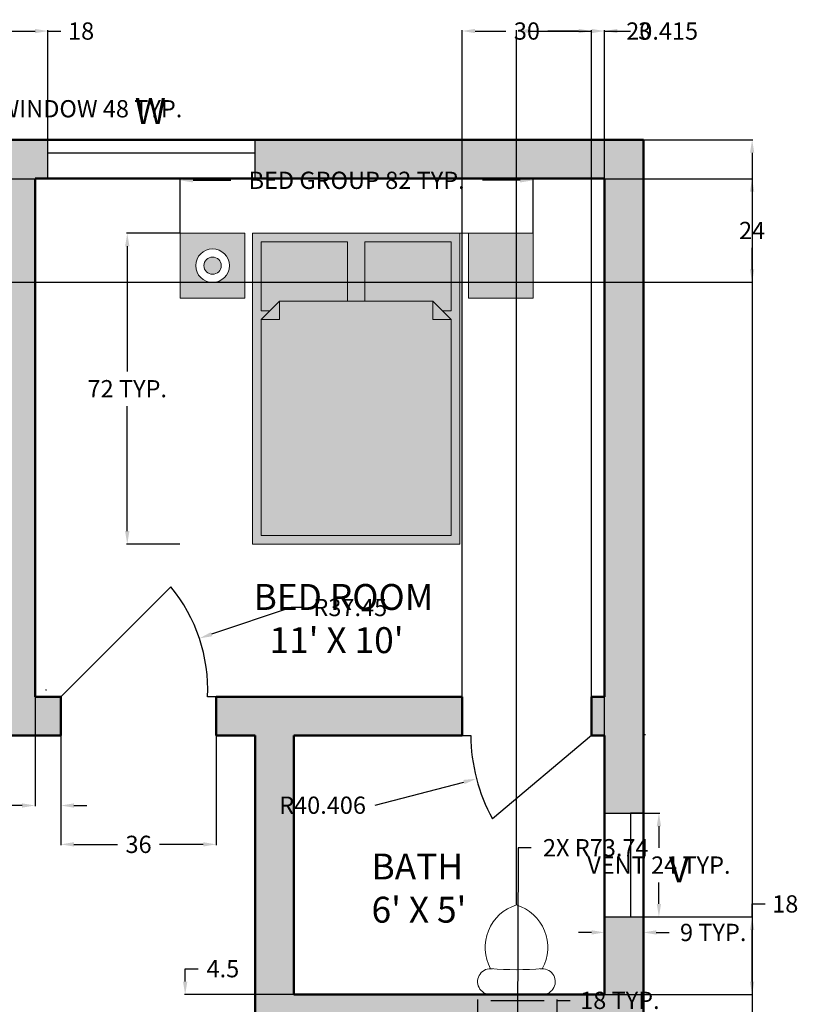
# Model space of a CAD drawing. Units: inches. Extents: x 30 to 385, y 81 to 626.
# Tile 4 of 4: x 204 to 385, y 398 to 626. Entities that reach past the tile are written whole.
import ezdxf

# ---------------------------------------------------------------- set-up
doc = ezdxf.new("R2010")
doc.units = ezdxf.units.IN
doc.header["$MEASUREMENT"] = 0
for name, color, linetype, lineweight in [('A-ANNO-DIMS', 2, 'Continuous', 18), ('A-ANNO-TEXT', 7, 'Continuous', 18), ('A-AREA-IDEN', 7, 'Continuous', 25), ('A-DOOR', 3, 'Continuous', 25), ('A-FLOR-FIXT', 8, 'Continuous', 18), ('A-FURN', 8, 'Continuous', 18), ('A-GLAZ', 4, 'Continuous', 25), ('A-WALL', 7, 'Continuous', 50), ('A-WALL-PATT', 32, 'Continuous', 13)]:
    doc.layers.add(name, color=color, linetype=linetype, lineweight=lineweight)
doc.layers.add('A-FURN-PATT', color=254, linetype='Continuous', lineweight=13, true_color=0xfeeab9)
doc.styles.get("Standard").update_dxf_attribs({"font": 'arial.ttf'})
doc.dimstyles.get("Standard").update_dxf_attribs({"dimtxt": 4, "dimasz": 3, "dimexe": 0.18, "dimexo": 0.0625, "dimgap": 2, "dimtad": 0, "dimtih": 1, "dimtoh": 1, "dimdec": 0, "dimzin": 0, "dimdsep": 46, "dimlunit": 3, "dimtxsty": 'Standard', "dimcen": 0.09, "dimadec": 0, "dimazin": 0, "dimtfac": 1, "dimtdec": 0, "dimtofl": 0, "dimtmove": 0, "dimatfit": 3, "dimfxl": 1, "dimtolj": 1, "dimtzin": 0, "dimarcsym": 0})

# ---------------------------------------------------------------- blocks, each defined once
blk = doc.blocks.new('WIN-48')
for p, q in [((0, 0), (0, 9)), ((48, 0), (48, 9)), ((0, 6), (48, 6))]:
    blk.add_line(p, q)
blk = doc.blocks.new('VENT-24')
for p, q in [((0, 0), (9, 0)), ((6, 0), (6, -24)), ((0, -24), (9, -24))]:
    blk.add_line(p, q)
blk = doc.blocks.new('WC-TANK')
blk.add_line((0, 0), (-12, 0.05))
for centre, radius, start, end in [((-12.01, -2.95), 3, 89.7749, 278.744), ((-0.01, -3), 3, 260.8057, 89.7749), ((-3.03, -10.92), 10.27, 151.067, 252.7388), ((-6.31, -79.48), 73.74, 85.108, 94.4417), ((-9.05, -10.9), 10.27, 286.8109, 28.4828)]:
    blk.add_arc(centre, radius, start, end)
blk = doc.blocks.new('BED-48X72-WITH-NIGHTSTANDS')
for p, q in [((48, 0), (50, 0)), ((2, -2), (22, -2)), ((2, -18), (2, -2)), ((22, -2), (22, -15.76)), ((26, -2), (46, -2)), ((26, -2), (26, -15.76)), ((46, -2), (46, -18)), ((2, -20), (6.24, -15.76)), ((41.76, -15.76), (6.24, -15.76)), ((6.24, -15.76), (6.24, -20)), ((46, -20), (41.76, -15.76)), ((41.76, -15.76), (41.76, -20)), ((2, -18), (4, -18)), ((44, -18), (46, -18)), ((2, -20), (6.24, -20)), ((2, -70), (2, -20)), ((41.76, -20), (46, -20)), ((46, -20), (46, -70)), ((46, -70), (2, -70))]:
    blk.add_line(p, q)
for points in [[(-16.78, 0), (-1.78, 0), (-1.78, -15), (-16.78, -15)], [(0, 0), (48, 0), (48, -72), (0, -72)], [(50, 0), (65, 0), (65, -15), (50, -15)]]:
    blk.add_lwpolyline(points, close=True)
for radius in [3.89, 3.89, 3.89, 2]:
    blk.add_circle((-9.28, -7.5), radius)
blk = doc.blocks.new('*D6')
at = {"layer": 'A-ANNO-DIMS', "color": 0, "lineweight": -2, "transparency": 16777216}
for p, q in [((144.92, 598.13), (144.92, 605.44)), ((147.92, 605.26), (189.92, 605.26)), ((192.92, 598.13), (192.92, 605.44)), ((192.92, 605.26), (195.92, 605.26))]:
    blk.add_line(p, q, dxfattribs=at)
at = {"layer": 'A-ANNO-DIMS', "color": 0, "transparency": 16777216}
for points in [[(147.92, 605.76), (147.92, 604.76), (144.92, 605.26)], [(189.92, 605.76), (189.92, 604.76), (192.92, 605.26)]]:
    blk.add_solid(points, dxfattribs=at)
at = {"layer": 'Defpoints', "color": 0, "transparency": 16777216}
for p in [(192.92, 605.26), (144.92, 598.06), (192.92, 598.06)]:
    blk.add_point(p, dxfattribs=at)
at = {"layer": 'A-ANNO-DIMS', "color": 0, "transparency": 16777216, "insert": (220.77, 605.26), "char_height": 4, "attachment_point": 5}
blk.add_mtext('\\A1;WINDOW 48 TYP.', dxfattribs=at)
blk = doc.blocks.new('*D8')
at = {"layer": 'A-ANNO-DIMS', "color": 0, "lineweight": -2, "transparency": 16777216}
for p, q in [((348.98, 442.06), (352.7, 442.06)), ((352.52, 439.06), (352.52, 434.07)), ((352.52, 421.06), (352.52, 426.05)), ((348.98, 418.06), (352.7, 418.06))]:
    blk.add_line(p, q, dxfattribs=at)
at = {"layer": 'A-ANNO-DIMS', "color": 0, "transparency": 16777216}
for points in [[(352.02, 439.06), (353.02, 439.06), (352.52, 442.06)], [(352.02, 421.06), (353.02, 421.06), (352.52, 418.06)]]:
    blk.add_solid(points, dxfattribs=at)
at = {"layer": 'Defpoints', "color": 0, "transparency": 16777216}
for p in [(348.92, 442.06), (352.52, 442.06), (348.92, 418.06)]:
    blk.add_point(p, dxfattribs=at)
at = {"layer": 'A-ANNO-DIMS', "color": 0, "transparency": 16777216, "insert": (352.52, 430.06), "char_height": 4, "attachment_point": 5}
blk.add_mtext('\\A1;VENT 24 TYP.', dxfattribs=at)
blk = doc.blocks.new('*D9')
at = {"layer": 'A-ANNO-DIMS', "color": 0, "lineweight": -2, "transparency": 16777216}
for p, q in [((339.92, 418), (339.92, 414.28)), ((348.92, 418), (348.92, 414.28)), ((336.92, 414.46), (333.92, 414.46)), ((351.92, 414.46), (354.92, 414.46))]:
    blk.add_line(p, q, dxfattribs=at)
at = {"layer": 'A-ANNO-DIMS', "color": 0, "transparency": 16777216}
for points in [[(336.92, 414.96), (336.92, 413.96), (339.92, 414.46)], [(351.92, 414.96), (351.92, 413.96), (348.92, 414.46)]]:
    blk.add_solid(points, dxfattribs=at)
at = {"layer": 'Defpoints', "color": 0, "transparency": 16777216}
for p in [(339.92, 418.06), (348.92, 418.06), (348.92, 414.46)]:
    blk.add_point(p, dxfattribs=at)
at = {"layer": 'A-ANNO-DIMS', "color": 0, "transparency": 16777216, "insert": (365.1, 414.46), "char_height": 4, "attachment_point": 5}
blk.add_mtext('\\A1;9 TYP.', dxfattribs=at)
blk = doc.blocks.new('*D11')
at = {"layer": 'A-ANNO-DIMS', "color": 0, "lineweight": -2, "transparency": 16777216}
for p, q in [((310.55, 395.68), (310.55, 398.91)), ((313.55, 398.73), (325.92, 398.73)), ((328.92, 395.68), (328.92, 398.91)), ((328.92, 398.73), (331.92, 398.73))]:
    blk.add_line(p, q, dxfattribs=at)
at = {"layer": 'A-ANNO-DIMS', "color": 0, "transparency": 16777216}
for points in [[(313.55, 399.23), (313.55, 398.23), (310.55, 398.73)], [(325.92, 399.23), (325.92, 398.23), (328.92, 398.73)]]:
    blk.add_solid(points, dxfattribs=at)
at = {"layer": 'Defpoints', "color": 0, "transparency": 16777216}
for p in [(328.92, 398.73), (310.55, 395.62), (328.92, 395.62)]:
    blk.add_point(p, dxfattribs=at)
at = {"layer": 'A-ANNO-DIMS', "color": 0, "transparency": 16777216, "insert": (343.47, 398.73), "char_height": 4, "attachment_point": 5}
blk.add_mtext('\\A1;18 TYP.', dxfattribs=at)
blk = doc.blocks.new('*D12')
at = {"layer": 'A-ANNO-DIMS', "color": 0, "lineweight": -2, "transparency": 16777216}
for p, q in [((241.57, 576.47), (241.57, 588.86)), ((244.57, 588.68), (253.27, 588.68)), ((320.35, 588.68), (311.65, 588.68)), ((323.35, 576.47), (323.35, 588.86))]:
    blk.add_line(p, q, dxfattribs=at)
at = {"layer": 'A-ANNO-DIMS', "color": 0, "transparency": 16777216}
for points in [[(244.57, 589.18), (244.57, 588.18), (241.57, 588.68)], [(320.35, 589.18), (320.35, 588.18), (323.35, 588.68)]]:
    blk.add_solid(points, dxfattribs=at)
at = {"layer": 'Defpoints', "color": 0, "transparency": 16777216}
for p in [(323.35, 588.68), (241.57, 576.41), (323.35, 576.41)]:
    blk.add_point(p, dxfattribs=at)
at = {"layer": 'A-ANNO-DIMS', "color": 0, "transparency": 16777216, "insert": (282.46, 588.68), "char_height": 4, "attachment_point": 5}
blk.add_mtext('\\A1;BED GROUP 82 TYP.', dxfattribs=at)
blk = doc.blocks.new('*D13')
at = {"layer": 'A-ANNO-DIMS', "color": 0, "lineweight": -2, "transparency": 16777216}
for p, q in [((241.51, 576.41), (229.12, 576.41)), ((229.3, 573.41), (229.3, 544.42)), ((229.3, 507.41), (229.3, 536.4)), ((241.51, 504.41), (229.12, 504.41))]:
    blk.add_line(p, q, dxfattribs=at)
at = {"layer": 'A-ANNO-DIMS', "color": 0, "transparency": 16777216}
for points in [[(228.8, 573.41), (229.8, 573.41), (229.3, 576.41)], [(228.8, 507.41), (229.8, 507.41), (229.3, 504.41)]]:
    blk.add_solid(points, dxfattribs=at)
at = {"layer": 'Defpoints', "color": 0, "transparency": 16777216}
for p in [(229.3, 576.41), (241.57, 576.41), (241.57, 504.41)]:
    blk.add_point(p, dxfattribs=at)
at = {"layer": 'A-ANNO-DIMS', "color": 0, "transparency": 16777216, "insert": (229.3, 540.41), "char_height": 4, "attachment_point": 5}
blk.add_mtext('\\A1;72 TYP.', dxfattribs=at)
blk = doc.blocks.new('*D17')
at = {"layer": 'A-ANNO-DIMS', "color": 0, "lineweight": -2, "transparency": 16777216}
for p, q in [((348.98, 598.06), (374.3, 598.06)), ((374.12, 595.06), (374.12, 357.61)), ((374.12, 112.06), (374.12, 349.52)), ((348.98, 109.06), (374.3, 109.06))]:
    blk.add_line(p, q, dxfattribs=at)
at = {"layer": 'A-ANNO-DIMS', "color": 0, "transparency": 16777216}
for points in [[(373.62, 595.06), (374.62, 595.06), (374.12, 598.06)], [(373.62, 112.06), (374.62, 112.06), (374.12, 109.06)]]:
    blk.add_solid(points, dxfattribs=at)
at = {"layer": 'Defpoints', "color": 0, "transparency": 16777216}
for p in [(348.92, 598.06), (374.12, 598.06), (348.92, 109.06)]:
    blk.add_point(p, dxfattribs=at)
at = {"layer": 'A-ANNO-DIMS', "color": 0, "transparency": 16777216, "insert": (374.12, 353.56), "char_height": 4, "attachment_point": 5}
blk.add_mtext('\\A1;489', dxfattribs=at)
blk = doc.blocks.new('*D22')
at = {"layer": 'A-ANNO-DIMS', "color": 0, "lineweight": -2, "transparency": 16777216}
for p, q in [((374.12, 418.06), (374.12, 421.06)), ((374.12, 421.06), (377.12, 421.06)), ((339.98, 418.06), (374.3, 418.06)), ((374.12, 403.06), (374.12, 415.06)), ((339.98, 400.06), (374.3, 400.06))]:
    blk.add_line(p, q, dxfattribs=at)
at = {"layer": 'A-ANNO-DIMS', "color": 0, "transparency": 16777216}
for points in [[(373.62, 415.06), (374.62, 415.06), (374.12, 418.06)], [(373.62, 403.06), (374.62, 403.06), (374.12, 400.06)]]:
    blk.add_solid(points, dxfattribs=at)
at = {"layer": 'Defpoints', "color": 0, "transparency": 16777216}
for p in [(339.92, 418.06), (374.12, 418.06), (339.92, 400.06)]:
    blk.add_point(p, dxfattribs=at)
at = {"layer": 'A-ANNO-DIMS', "color": 0, "transparency": 16777216, "insert": (381.8, 421.06), "char_height": 4, "attachment_point": 5}
blk.add_mtext('\\A1;18', dxfattribs=at)
blk = doc.blocks.new('*D27')
at = {"layer": 'A-ANNO-DIMS', "color": 0, "lineweight": -2, "transparency": 16777216}
for p, q in [((192.92, 598.13), (192.92, 623.44)), ((195.92, 623.26), (207.92, 623.26)), ((210.92, 598.13), (210.92, 623.44)), ((210.92, 623.26), (213.92, 623.26))]:
    blk.add_line(p, q, dxfattribs=at)
at = {"layer": 'A-ANNO-DIMS', "color": 0, "transparency": 16777216}
for points in [[(195.92, 623.76), (195.92, 622.76), (192.92, 623.26)], [(207.92, 623.76), (207.92, 622.76), (210.92, 623.26)]]:
    blk.add_solid(points, dxfattribs=at)
at = {"layer": 'Defpoints', "color": 0, "transparency": 16777216}
for p in [(210.92, 623.26), (192.92, 598.06), (210.92, 598.06)]:
    blk.add_point(p, dxfattribs=at)
at = {"layer": 'A-ANNO-DIMS', "color": 0, "transparency": 16777216, "insert": (218.6, 623.26), "char_height": 4, "attachment_point": 5}
blk.add_mtext('\\A1;18', dxfattribs=at)
blk = doc.blocks.new('*D29')
at = {"layer": 'A-ANNO-DIMS', "color": 0, "lineweight": -2, "transparency": 16777216}
for p, q in [((198.98, 589.06), (374.3, 589.06)), ((374.12, 586.06), (374.12, 581.07)), ((374.12, 568.06), (374.12, 573.06)), ((198.98, 565.06), (374.3, 565.06))]:
    blk.add_line(p, q, dxfattribs=at)
at = {"layer": 'A-ANNO-DIMS', "color": 0, "transparency": 16777216}
for points in [[(373.62, 586.06), (374.62, 586.06), (374.12, 589.06)], [(373.62, 568.06), (374.62, 568.06), (374.12, 565.06)]]:
    blk.add_solid(points, dxfattribs=at)
at = {"layer": 'Defpoints', "color": 0, "transparency": 16777216}
for p in [(198.92, 589.06), (374.12, 589.06), (198.92, 565.06)]:
    blk.add_point(p, dxfattribs=at)
at = {"layer": 'A-ANNO-DIMS', "color": 0, "transparency": 16777216, "insert": (374.12, 577.06), "char_height": 4, "attachment_point": 5}
blk.add_mtext('\\A1;24', dxfattribs=at)
blk = doc.blocks.new('*D34')
at = {"layer": 'A-ANNO-DIMS', "color": 0, "lineweight": -2, "transparency": 16777216}
for p, q in [((213.92, 460), (213.92, 434.68)), ((249.92, 460), (249.92, 434.68)), ((216.92, 434.86), (227.06, 434.86)), ((246.92, 434.86), (236.78, 434.86))]:
    blk.add_line(p, q, dxfattribs=at)
at = {"layer": 'A-ANNO-DIMS', "color": 0, "transparency": 16777216}
for points in [[(216.92, 435.36), (216.92, 434.36), (213.92, 434.86)], [(246.92, 435.36), (246.92, 434.36), (249.92, 434.86)]]:
    blk.add_solid(points, dxfattribs=at)
at = {"layer": 'Defpoints', "color": 0, "transparency": 16777216}
for p in [(213.92, 460.06), (249.92, 460.06), (213.92, 434.86)]:
    blk.add_point(p, dxfattribs=at)
at = {"layer": 'A-ANNO-DIMS', "color": 0, "transparency": 16777216, "insert": (231.92, 434.86), "char_height": 4, "attachment_point": 5}
blk.add_mtext('\\A1;36', dxfattribs=at)
blk = doc.blocks.new('*D35')
at = {"layer": 'A-ANNO-DIMS', "color": 0, "lineweight": -2, "transparency": 16777216}
for p, q in [((207.92, 469), (207.92, 443.68)), ((213.92, 469), (213.92, 443.68)), ((204.92, 443.86), (201.92, 443.86)), ((216.92, 443.86), (219.92, 443.86))]:
    blk.add_line(p, q, dxfattribs=at)
at = {"layer": 'A-ANNO-DIMS', "color": 0, "transparency": 16777216}
for points in [[(204.92, 444.36), (204.92, 443.36), (207.92, 443.86)], [(216.92, 444.36), (216.92, 443.36), (213.92, 443.86)]]:
    blk.add_solid(points, dxfattribs=at)
at = {"layer": 'Defpoints', "color": 0, "transparency": 16777216}
for p in [(207.92, 469.06), (213.92, 469.06), (207.92, 443.86)]:
    blk.add_point(p, dxfattribs=at)
at = {"layer": 'A-ANNO-DIMS', "color": 0, "transparency": 16777216, "insert": (198.6, 443.86), "char_height": 4, "attachment_point": 5}
blk.add_mtext('\\A1;6', dxfattribs=at)
blk = doc.blocks.new('*D38')
at = {"layer": 'A-ANNO-DIMS', "color": 0, "lineweight": -2, "transparency": 16777216}
for p, q in [((306.92, 460.13), (306.92, 623.44)), ((309.92, 623.26), (317.06, 623.26)), ((333.92, 623.26), (326.78, 623.26)), ((336.92, 460.13), (336.92, 623.44))]:
    blk.add_line(p, q, dxfattribs=at)
at = {"layer": 'A-ANNO-DIMS', "color": 0, "transparency": 16777216}
for points in [[(309.92, 623.76), (309.92, 622.76), (306.92, 623.26)], [(333.92, 623.76), (333.92, 622.76), (336.92, 623.26)]]:
    blk.add_solid(points, dxfattribs=at)
at = {"layer": 'Defpoints', "color": 0, "transparency": 16777216}
for p in [(336.92, 623.26), (306.92, 460.06), (336.92, 460.06)]:
    blk.add_point(p, dxfattribs=at)
at = {"layer": 'A-ANNO-DIMS', "color": 0, "transparency": 16777216, "insert": (321.92, 623.26), "char_height": 4, "attachment_point": 5}
blk.add_mtext('\\A1;30', dxfattribs=at)
blk = doc.blocks.new('*D39')
at = {"layer": 'A-ANNO-DIMS', "color": 0, "lineweight": -2, "transparency": 16777216}
for p, q in [((333.92, 623.26), (330.92, 623.26)), ((336.92, 460.13), (336.92, 623.44)), ((339.92, 460.13), (339.92, 623.44)), ((342.92, 623.26), (345.92, 623.26))]:
    blk.add_line(p, q, dxfattribs=at)
at = {"layer": 'A-ANNO-DIMS', "color": 0, "transparency": 16777216}
for points in [[(333.92, 623.76), (333.92, 622.76), (336.92, 623.26)], [(342.92, 623.76), (342.92, 622.76), (339.92, 623.26)]]:
    blk.add_solid(points, dxfattribs=at)
at = {"layer": 'Defpoints', "color": 0, "transparency": 16777216}
for p in [(339.92, 623.26), (336.92, 460.06), (339.92, 460.06)]:
    blk.add_point(p, dxfattribs=at)
at = {"layer": 'A-ANNO-DIMS', "color": 0, "transparency": 16777216, "insert": (349.23, 623.26), "char_height": 4, "attachment_point": 5}
blk.add_mtext('\\A1;3', dxfattribs=at)
blk = doc.blocks.new('*D41')
at = {"layer": 'A-ANNO-DIMS', "color": 0, "lineweight": -2, "transparency": 16777216}
for p, q in [((242.72, 403.06), (242.72, 406.06)), ((242.72, 406.06), (245.72, 406.06)), ((267.86, 400.06), (242.54, 400.06)), ((267.86, 395.56), (242.54, 395.56)), ((242.72, 392.56), (242.72, 389.56))]:
    blk.add_line(p, q, dxfattribs=at)
at = {"layer": 'A-ANNO-DIMS', "color": 0, "transparency": 16777216}
for points in [[(242.22, 403.06), (243.22, 403.06), (242.72, 400.06)], [(242.22, 392.56), (243.22, 392.56), (242.72, 395.56)]]:
    blk.add_solid(points, dxfattribs=at)
at = {"layer": 'Defpoints', "color": 0, "transparency": 16777216}
for p in [(242.72, 400.06), (267.92, 400.06), (267.92, 395.56)]:
    blk.add_point(p, dxfattribs=at)
at = {"layer": 'A-ANNO-DIMS', "color": 0, "transparency": 16777216, "insert": (251.46, 406.06), "char_height": 4, "attachment_point": 5}
blk.add_mtext('\\A1;4.5', dxfattribs=at)
blk = doc.blocks.new('*D42')
at = {"layer": 'A-ANNO-DIMS', "color": 0, "lineweight": -2, "transparency": 16777216}
for p, q in [((319.5, 420.88), (319.5, 623.44)), ((322.5, 623.26), (336.92, 623.26)), ((339.92, 418.13), (339.92, 623.44)), ((339.92, 623.26), (342.92, 623.26))]:
    blk.add_line(p, q, dxfattribs=at)
at = {"layer": 'A-ANNO-DIMS', "color": 0, "transparency": 16777216}
for points in [[(322.5, 623.76), (322.5, 622.76), (319.5, 623.26)], [(336.92, 623.76), (336.92, 622.76), (339.92, 623.26)]]:
    blk.add_solid(points, dxfattribs=at)
at = {"layer": 'Defpoints', "color": 0, "transparency": 16777216}
for p in [(339.92, 623.26), (319.5, 420.82), (339.92, 418.06)]:
    blk.add_point(p, dxfattribs=at)
at = {"layer": 'A-ANNO-DIMS', "color": 0, "transparency": 16777216, "insert": (353.27, 623.26), "char_height": 4, "attachment_point": 5}
blk.add_mtext('\\A1;20.415', dxfattribs=at)
blk = doc.blocks.new('*D56')
at = {"layer": 'A-ANNO-DIMS', "color": 0, "lineweight": -2, "transparency": 16777216}
for p, q in [((267.31, 489.73), (248.85, 483.54)), ((270.31, 489.73), (267.31, 489.73)), ((210.41, 470.67), (210.59, 470.67)), ((210.5, 470.58), (210.5, 470.76))]:
    blk.add_line(p, q, dxfattribs=at)
at = {"layer": 'A-ANNO-DIMS', "color": 0, "transparency": 16777216}
blk.add_solid([(248.69, 484.01), (249.01, 483.06), (246.01, 482.58)], dxfattribs=at)
at = {"layer": 'Defpoints', "color": 0, "transparency": 16777216}
for p in [(246.01, 482.58), (210.5, 470.67)]:
    blk.add_point(p, dxfattribs=at)
at = {"layer": 'A-ANNO-DIMS', "color": 0, "transparency": 16777216, "insert": (280.99, 489.73), "char_height": 4, "attachment_point": 5}
blk.add_mtext('\\A1;R37.45', dxfattribs=at)
blk = doc.blocks.new('*D58')
at = {"layer": 'A-ANNO-DIMS', "color": 0, "lineweight": -2, "transparency": 16777216}
for p, q in [((349.23, 460.28), (349.41, 460.28)), ((349.32, 460.19), (349.32, 460.37)), ((286.78, 443.93), (307.33, 449.3))]:
    blk.add_line(p, q, dxfattribs=at)
at = {"layer": 'A-ANNO-DIMS', "color": 0, "transparency": 16777216}
blk.add_solid([(307.2, 449.79), (307.46, 448.82), (310.23, 450.06)], dxfattribs=at)
at = {"layer": 'Defpoints', "color": 0, "transparency": 16777216}
for p in [(349.32, 460.28), (310.23, 450.06)]:
    blk.add_point(p, dxfattribs=at)
at = {"layer": 'A-ANNO-DIMS', "color": 0, "transparency": 16777216, "insert": (274.56, 443.93), "char_height": 4, "attachment_point": 5}
blk.add_mtext('\\A1;R40.406', dxfattribs=at)
blk = doc.blocks.new('*D59')
at = {"layer": 'A-ANNO-DIMS', "color": 0, "lineweight": -2, "transparency": 16777216}
for p, q in [((319.9, 434.08), (319.73, 392.83)), ((322.9, 434.08), (319.9, 434.08)), ((319.34, 316.09), (319.52, 316.09)), ((319.43, 316), (319.43, 316.18))]:
    blk.add_line(p, q, dxfattribs=at)
at = {"layer": 'A-ANNO-DIMS', "color": 0, "transparency": 16777216}
blk.add_solid([(319.23, 392.83), (320.23, 392.83), (319.72, 389.83)], dxfattribs=at)
at = {"layer": 'Defpoints', "color": 0, "transparency": 16777216}
for p in [(319.72, 389.83), (319.43, 316.09)]:
    blk.add_point(p, dxfattribs=at)
at = {"layer": 'A-ANNO-DIMS', "color": 0, "transparency": 16777216, "insert": (337.88, 434.08), "char_height": 4, "attachment_point": 5}
blk.add_mtext('\\A1;2X R73.74', dxfattribs=at)

msp = doc.modelspace()

# ---------------------------------------------------------------- hatches: boundary and pattern name
at = {"layer": 'A-FURN-PATT'}
h = msp.add_hatch(color=256, dxfattribs=at)
h.paths.add_polyline_path([(306.3516, 576.4124), (258.3516, 576.4124), (258.3516, 504.4124), (306.3516, 504.4124)])
h.paths.add_polyline_path([(260.3516, 558.4124), (260.3516, 574.4124), (280.3516, 574.4124), (280.3516, 560.655), (284.3516, 560.655), (284.3516, 574.4124), (304.3516, 574.4124), (304.3516, 558.4124), (302.3516, 558.4124), (304.3516, 556.4124), (304.3516, 506.4124), (260.3516, 506.4124), (260.3516, 556.4124), (262.3516, 558.4124)], flags=16)
h.paths.add_polyline_path([(323.3516, 576.4124), (308.3516, 576.4124), (308.3516, 561.4124), (323.3516, 561.4124)])
h.paths.add_polyline_path([(256.5684, 576.4124), (241.5684, 576.4124), (241.5684, 561.4124), (256.5684, 561.4124)])
h.paths.add_polyline_path([(245.177, 568.9124, -1), (252.9599, 568.9124, -1)], flags=16)
h.paths.add_polyline_path([(247.0684, 568.9124, -1), (251.0684, 568.9124, -1)], flags=0)
h = msp.add_hatch(color=256, dxfattribs=at)
h.paths.add_polyline_path([(280.3516, 574.4124), (260.3516, 574.4124), (260.3516, 558.4124), (262.3516, 558.4124), (264.5942, 560.655), (280.3516, 560.655)])
h.paths.add_polyline_path([(304.3516, 574.4124), (284.3516, 574.4124), (284.3516, 560.655), (300.109, 560.655), (302.3516, 558.4124), (304.3516, 558.4124)])
h = msp.add_hatch(color=256, dxfattribs=at)
h.paths.add_polyline_path([(304.3516, 556.4124), (300.109, 556.4124), (300.109, 560.655), (264.5942, 560.655), (264.5942, 556.4124), (260.3516, 556.4124), (260.3516, 506.4124), (304.3516, 506.4124)])
h.paths.add_polyline_path([(300.109, 560.655), (300.109, 556.4124), (304.3516, 556.4124)], flags=17)
h.paths.add_polyline_path([(264.5942, 560.655), (260.3516, 556.4124), (264.5942, 556.4124)], flags=17)
at = {"layer": 'A-WALL-PATT'}
h = msp.add_hatch(color=256, dxfattribs=at)
h.paths.add_polyline_path([(156.9551, 469.0638), (66.919, 469.0638), (66.919, 472.0638), (57.919, 472.0638), (57.919, 433.0638), (66.919, 433.0638), (66.919, 460.0638), (156.9551, 460.0638)])
h.paths.add_polyline_path([(207.919, 589.0638), (210.919, 589.0638), (210.919, 598.0638), (192.919, 598.0638), (192.919, 589.0638), (198.919, 589.0638), (198.919, 469.0638), (192.9551, 469.0638), (192.9551, 460.0638), (213.919, 460.0638), (213.919, 469.0638), (207.919, 469.0638)])
h.paths.add_polyline_path([(348.919, 598.0638), (258.919, 598.0638), (258.919, 589.0638), (339.919, 589.0638), (339.919, 469.0638), (336.919, 469.0638), (336.919, 460.0638), (339.919, 460.0638), (339.919, 442.0638), (348.919, 442.0638)])
h = msp.add_hatch(color=256, dxfattribs=at)
h.paths.add_polyline_path([(66.919, 385.0638), (57.919, 385.0638), (57.919, 331.0638), (60.919, 331.0638), (66.919, 331.0638)])
h.paths.add_polyline_path([(306.919, 469.0638), (249.919, 469.0638), (249.919, 460.0638), (258.919, 460.0638), (258.919, 392.5638), (267.919, 392.5638), (267.919, 395.5638), (339.919, 395.5638), (339.919, 377.5638), (348.919, 377.5638), (348.919, 418.0638), (339.919, 418.0638), (339.919, 400.0638), (267.919, 400.0638), (267.919, 460.0638), (306.919, 460.0638)])
h.paths.add_polyline_path([(339.919, 194.5638), (207.919, 194.5638), (207.919, 326.5638), (210.919, 326.5638), (210.919, 335.5638), (198.919, 335.5638), (198.919, 256.0638), (195.919, 256.0638), (195.919, 247.0638), (198.919, 247.0638), (198.919, 194.5638), (198.919, 185.5638), (339.919, 185.5638)])

# ---------------------------------------------------------------- linework, layer by layer
at = {"layer": 'A-DOOR'}
for p, q in [((213.919, 469.0638), (239.3749, 494.5197)), ((249.919, 469.0638), (247.919, 469.0638)), ((306.919, 460.0638), (308.919, 460.0638)), ((336.919, 460.0638), (313.9377, 440.7802))]:
    msp.add_line(p, q, dxfattribs=at)
for centre, radius, start, end in [((210.5049, 470.6678), 37.4484, 357.545243, 39.563015), ((349.3243, 460.2847), 40.4059, 180.313109, 208.862725)]:
    msp.add_arc(centre, radius, start, end, dxfattribs=at)
at = {"layer": 'A-GLAZ'}
msp.add_line((348.919, 442.0638), (345.919, 442.0638), dxfattribs=at)
at = {"layer": 'A-WALL'}
for p, q in [((348.919, 598.0638), (57.919, 598.0638)), ((348.919, 109.0638), (348.919, 598.0638)), ((339.919, 589.0638), (207.919, 589.0638)), ((207.919, 469.0638), (207.919, 589.0638)), ((207.919, 469.0638), (207.919, 589.0638)), ((339.919, 469.0638), (339.919, 589.0638)), ((213.919, 469.0638), (207.919, 469.0638)), ((213.919, 469.0638), (213.919, 460.0638)), ((249.919, 469.0638), (249.919, 460.0638)), ((306.919, 469.0638), (249.919, 469.0638)), ((306.919, 469.0638), (306.919, 460.0638)), ((339.919, 469.0638), (336.919, 469.0638)), ((336.919, 469.0638), (336.919, 460.0638)), ((213.919, 460.0638), (192.9551, 460.0638)), ((258.919, 460.0638), (249.919, 460.0638)), ((258.919, 392.5638), (258.919, 460.0638)), ((267.919, 400.0638), (267.919, 460.0638)), ((306.919, 460.0638), (267.919, 460.0638)), ((339.919, 460.0638), (336.919, 460.0638)), ((339.919, 400.0638), (339.919, 460.0638)), ((339.919, 400.0638), (267.919, 400.0638))]:
    msp.add_line(p, q, dxfattribs=at)

# ---------------------------------------------------------------- block references
at = {"layer": 'A-FLOR-FIXT', "rotation": 180.2251261579}
msp.add_blockref('WC-TANK', (313.5035, 400.0638), dxfattribs=at)
at = {"layer": 'A-FURN'}
msp.add_blockref('BED-48X72-WITH-NIGHTSTANDS', (258.3516, 576.4124), dxfattribs=at)
at = {"layer": 'A-GLAZ'}
for name, p in [('WIN-48', (210.919, 589.0638)), ('VENT-24', (339.919, 442.0638))]:
    msp.add_blockref(name, p, dxfattribs=at)

# ---------------------------------------------------------------- texts
at = {"layer": 'A-ANNO-TEXT', "char_height": 6, "attachment_point": 1}
for s, insert in [('W', (231.0641, 607.7328)), ('V', (354.8225, 432.0466))]:
    msp.add_mtext_dynamic_manual_height_columns(s, width=76.086845, gutter_width=1, heights=[0], dxfattribs=dict(at, insert=insert))
at = {"layer": 'A-AREA-IDEN', "char_height": 6, "attachment_point": 1}
for s, insert in [("BED ROOM\\P  11' X 10'", (258.5909, 495.1674)), ("  BATH\\P  6' X 5'", (282.2434, 432.7242))]:
    msp.add_mtext_dynamic_manual_height_columns(s, width=76.086845, gutter_width=1, heights=[0], dxfattribs=dict(at, insert=insert))

# ---------------------------------------------------------------- dimensions: what is measured, and where the dimension line sits
at = {"layer": 'A-ANNO-DIMS'}
for base, p1, p2, override, picture, middle in [((210.919, 623.2638), (192.919, 598.0638), (210.919, 598.0638), {"dimdec": 0, "dimlfac": 1, "dimrnd": 0, "dimzin": 0, "dimdsep": 46, "dimlunit": 2}, '*D27', (218.5998, 623.2638)), ((336.919, 623.2638), (306.919, 460.0638), (336.919, 460.0638), {"dimdec": 0, "dimlfac": 1, "dimrnd": 0, "dimzin": 0, "dimdsep": 46, "dimlunit": 2}, '*D38', (321.919, 623.2638)), ((339.919029, 623.263849), (319.503535, 420.819359), (339.919029, 418.063849), {"dimdec": 3, "dimlfac": 1, "dimrnd": 0, "dimzin": 0, "dimdsep": 46, "dimlunit": 2}, '*D42', (353.271007, 623.263849)), ((339.919, 623.2638), (336.919, 460.0638), (339.919, 460.0638), {"dimdec": 0, "dimlfac": 1, "dimrnd": 0, "dimzin": 0, "dimdsep": 46, "dimlunit": 2}, '*D39', (349.2287, 623.2638))]:
    dim = msp.add_linear_dim(base=base, p1=p1, p2=p2, dimstyle='Standard', override=override, dxfattribs=at)
    dim.commit()
    dim.dimension.update_dxf_attribs({"geometry": picture, "text_midpoint": middle})
for base, p1, p2, text, picture, middle in [((192.919, 605.2638), (144.919, 598.0638), (192.919, 598.0638), 'WINDOW <> TYP.', '*D6', (220.7717, 605.2638)), ((323.3516, 588.6799), (241.5684, 576.4124), (323.3516, 576.4124), 'BED GROUP <> TYP.', '*D12', (282.46, 588.6799)), ((348.919, 414.4638), (339.919, 418.0638), (348.919, 418.0638), '<> TYP.', '*D9', (365.1005, 414.4638)), ((328.9197, 398.7329), (310.5498, 395.6154), (328.9197, 395.6154), '<> TYP.', '*D11', (343.4668, 398.7329))]:
    dim = msp.add_linear_dim(base=base, p1=p1, p2=p2, text=text, dimstyle='Standard', override={"dimdec": 0, "dimlfac": 1, "dimrnd": 0, "dimzin": 0, "dimdsep": 46, "dimlunit": 2}, dxfattribs=at)
    dim.commit()
    dim.dimension.update_dxf_attribs({"geometry": picture, "text_midpoint": middle})
for base, p1, p2, angle, override, picture, middle in [((374.119, 598.0638), (348.919, 109.0638), (348.919, 598.0638), 90, {"dimdec": 0, "dimlfac": 1, "dimrnd": 0, "dimzin": 0, "dimdsep": 46, "dimlunit": 2}, '*D17', (374.119, 353.5638)), ((374.119, 589.0638), (198.919, 565.0638), (198.919, 589.0638), 90, {"dimdec": 0, "dimlfac": 1, "dimrnd": 0, "dimzin": 0, "dimdsep": 46, "dimlunit": 2}, '*D29', (374.119, 577.0638)), ((207.919, 443.8638), (213.919, 469.0638), (207.919, 469.0638), 180, {"dimdec": 0, "dimlfac": 1, "dimrnd": 0, "dimzin": 0, "dimdsep": 46, "dimlunit": 2}, '*D35', (198.5984, 443.8638)), ((213.919, 434.8638), (249.919, 460.0638), (213.919, 460.0638), 180, {"dimdec": 0, "dimlfac": 1, "dimrnd": 0, "dimzin": 0, "dimdsep": 46, "dimlunit": 2}, '*D34', (231.919, 434.8638)), ((374.119, 418.0638), (339.919, 400.0638), (339.919, 418.0638), 90, {"dimdec": 0, "dimlfac": 1, "dimrnd": 0, "dimzin": 0, "dimdsep": 46, "dimlunit": 2}, '*D22', (381.7998, 421.0638)), ((242.719, 400.0638), (267.919, 395.5638), (267.919, 400.0638), 90, {"dimdec": 1, "dimlfac": 1, "dimrnd": 0, "dimzin": 0, "dimdsep": 46, "dimlunit": 2}, '*D41', (251.4557, 406.0638))]:
    dim = msp.add_linear_dim(base=base, p1=p1, p2=p2, angle=angle, dimstyle='Standard', override=override, dxfattribs=at)
    dim.commit()
    dim.dimension.update_dxf_attribs({"geometry": picture, "text_midpoint": middle})
for base, p1, p2, text, picture, middle in [((229.3009, 576.4124), (241.5684, 504.4124), (241.5684, 576.4124), '<> TYP.', '*D13', (229.3009, 540.4124)), ((352.519, 442.0638), (348.919, 418.0638), (348.919, 442.0638), 'VENT <> TYP.', '*D8', (352.519, 430.0638))]:
    dim = msp.add_linear_dim(base=base, p1=p1, p2=p2, angle=90, text=text, dimstyle='Standard', override={"dimdec": 0, "dimlfac": 1, "dimrnd": 0, "dimzin": 0, "dimdsep": 46, "dimlunit": 2}, dxfattribs=at)
    dim.commit()
    dim.dimension.update_dxf_attribs({"geometry": picture, "text_midpoint": middle})
for center, mpoint, override, picture, middle in [((210.5049, 470.6678), (246.0069, 482.584), {"dimdec": 2, "dimlfac": 1, "dimrnd": 0, "dimzin": 0, "dimdsep": 46, "dimlunit": 2}, '*D56', (280.9862, 489.7337)), ((349.3243, 460.2847), (310.2332, 450.061), {"dimdec": 3, "dimlfac": 1, "dimrnd": 0, "dimzin": 0, "dimdsep": 46, "dimlunit": 2}, '*D58', (286.7786, 443.9268))]:
    dim = msp.add_radius_dim(center=center, mpoint=mpoint, dimstyle='Standard', override=override, dxfattribs=at)
    dim.commit()
    dim.dimension.update_dxf_attribs({"geometry": picture, "text_midpoint": middle, "dimtype": 164})
dim = msp.add_radius_dim(center=(319.4328, 316.0876), mpoint=(319.723, 389.832), text='2X <>', dimstyle='Standard', override={"dimdec": 2, "dimlfac": 1, "dimrnd": 0, "dimzin": 0, "dimdsep": 46, "dimlunit": 2}, dxfattribs=at)
dim.commit()
dim.dimension.update_dxf_attribs({"geometry": '*D59', "text_midpoint": (337.8835, 434.0786), "dimtype": 164})

doc.saveas('drawing.dxf')
